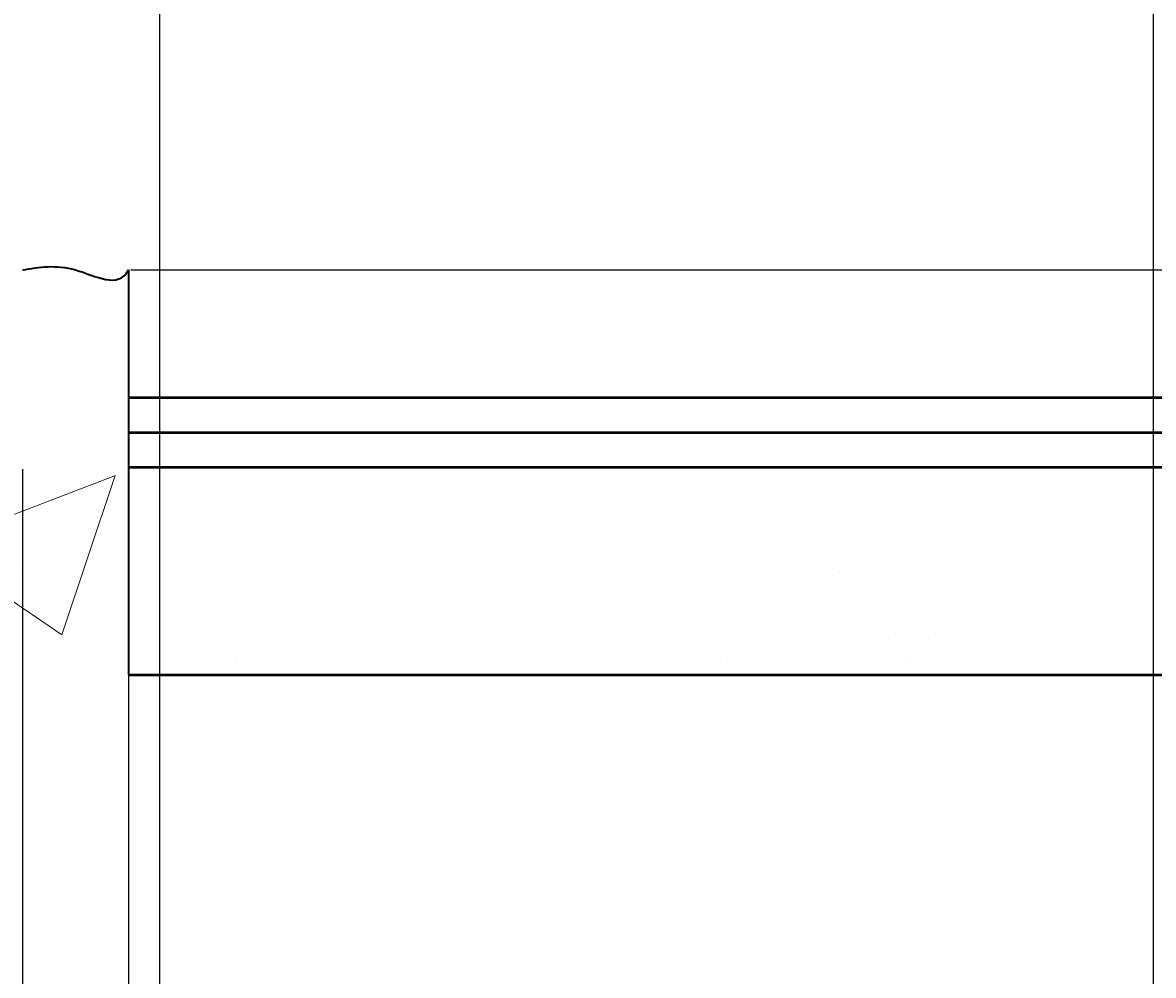
# Model space of a CAD drawing. Units: inches. Extents: x 2812 to 3051, y 1398 to 1659.
# Tile 10 of 65: x 2848 to 2880, y 1473 to 1501. Entities that reach past the tile are written whole.
import ezdxf

# ---------------------------------------------------------------- set-up
doc = ezdxf.new("R2010")
doc.units = ezdxf.units.IN
for name, color, linetype, lineweight in [('A-ANNO-DIMS', 2, 'Continuous', 18), ('P-SANR-PIPE', 4, 'Continuous', 35), ('S-CONC', 7, 'Continuous', 50), ('S-CONC-PATT', 8, 'Continuous', 18)]:
    doc.layers.add(name, color=color, linetype=linetype, lineweight=lineweight)
doc.styles.get("Standard").update_dxf_attribs({"font": 'arial.ttf'})
doc.dimstyles.get("Standard").update_dxf_attribs({"dimtxt": 0.18, "dimasz": 0.18, "dimexe": 0.18, "dimexo": 0.0625, "dimgap": 0.09, "dimtad": 0, "dimtih": 1, "dimtoh": 1, "dimdec": 4, "dimzin": 0, "dimdsep": 46, "dimtxsty": 'Standard', "dimcen": 0.09, "dimadec": 0, "dimazin": 0, "dimtfac": 1, "dimtdec": 4, "dimtofl": 0, "dimtmove": 0, "dimatfit": 3, "dimfxl": 1, "dimtolj": 1, "dimtzin": 0, "dimarcsym": 0})

# ---------------------------------------------------------------- blocks, each defined once
blk = doc.blocks.new('*D28')
at = {"layer": 'A-ANNO-DIMS', "color": 0, "lineweight": -2, "transparency": 16777216}
for p, q in [((2851.646, 1598.667), (2851.646, 1397.505)), ((2844.385, 1559.757), (2844.385, 1397.505)), ((2844.565, 1397.685), (2847.64, 1397.685)), ((2851.466, 1397.685), (2848.391, 1397.685))]:
    blk.add_line(p, q, dxfattribs=at)
at = {"layer": 'A-ANNO-DIMS', "color": 0, "transparency": 16777216}
for points in [[(2844.565, 1397.715), (2844.565, 1397.655), (2844.385, 1397.685)], [(2851.466, 1397.715), (2851.466, 1397.655), (2851.646, 1397.685)]]:
    blk.add_solid(points, dxfattribs=at)
at = {"layer": 'Defpoints', "color": 0, "transparency": 16777216}
for p in [(2851.646, 1598.73), (2844.385, 1559.82), (2851.646, 1397.685)]:
    blk.add_point(p, dxfattribs=at)
at = {"layer": 'A-ANNO-DIMS', "color": 0, "transparency": 16777216, "insert": (2848.016, 1397.685), "char_height": 0.18, "attachment_point": 5}
blk.add_mtext('\\A1;7.261', dxfattribs=at)
blk = doc.blocks.new('*D42')
at = {"layer": 'A-ANNO-DIMS', "color": 0, "lineweight": -2, "transparency": 16777216}
for p, q in [((2828.385, 1489.973), (2828.385, 1397.505)), ((2847.686, 1487.973), (2847.686, 1397.505)), ((2828.565, 1397.685), (2837.72, 1397.685)), ((2847.506, 1397.685), (2838.351, 1397.685))]:
    blk.add_line(p, q, dxfattribs=at)
at = {"layer": 'A-ANNO-DIMS', "color": 0, "transparency": 16777216}
for points in [[(2828.565, 1397.715), (2828.565, 1397.655), (2828.385, 1397.685)], [(2847.506, 1397.715), (2847.506, 1397.655), (2847.686, 1397.685)]]:
    blk.add_solid(points, dxfattribs=at)
at = {"layer": 'Defpoints', "color": 0, "transparency": 16777216}
for p in [(2828.385, 1490.035), (2847.686, 1488.035), (2847.686, 1397.685)]:
    blk.add_point(p, dxfattribs=at)
at = {"layer": 'A-ANNO-DIMS', "color": 0, "transparency": 16777216, "insert": (2838.036, 1397.685), "char_height": 0.18, "attachment_point": 5}
blk.add_mtext('\\A1;19.3', dxfattribs=at)
blk = doc.blocks.new('*D43')
at = {"layer": 'A-ANNO-DIMS', "color": 0, "lineweight": -2, "transparency": 16777216}
for p, q in [((2847.686, 1487.973), (2847.686, 1397.505)), ((2850.748, 1487.973), (2850.748, 1397.505)), ((2847.866, 1397.685), (2848.825, 1397.685)), ((2850.568, 1397.685), (2849.61, 1397.685))]:
    blk.add_line(p, q, dxfattribs=at)
at = {"layer": 'A-ANNO-DIMS', "color": 0, "transparency": 16777216}
for points in [[(2847.866, 1397.715), (2847.866, 1397.655), (2847.686, 1397.685)], [(2850.568, 1397.715), (2850.568, 1397.655), (2850.748, 1397.685)]]:
    blk.add_solid(points, dxfattribs=at)
at = {"layer": 'Defpoints', "color": 0, "transparency": 16777216}
for p in [(2847.686, 1488.035), (2850.748, 1488.035), (2850.748, 1397.685)]:
    blk.add_point(p, dxfattribs=at)
at = {"layer": 'A-ANNO-DIMS', "color": 0, "transparency": 16777216, "insert": (2849.217, 1397.685), "char_height": 0.18, "attachment_point": 5}
blk.add_mtext('\\A1;3.062', dxfattribs=at)
blk = doc.blocks.new('*D44')
at = {"layer": 'A-ANNO-DIMS', "color": 0, "lineweight": -2, "transparency": 16777216}
for p, q in [((2850.748, 1487.973), (2850.748, 1397.505)), ((2896.385, 1487.973), (2896.385, 1397.505)), ((2850.928, 1397.685), (2873.17, 1397.685)), ((2896.205, 1397.685), (2873.964, 1397.685))]:
    blk.add_line(p, q, dxfattribs=at)
at = {"layer": 'A-ANNO-DIMS', "color": 0, "transparency": 16777216}
for points in [[(2850.928, 1397.715), (2850.928, 1397.655), (2850.748, 1397.685)], [(2896.205, 1397.715), (2896.205, 1397.655), (2896.385, 1397.685)]]:
    blk.add_solid(points, dxfattribs=at)
at = {"layer": 'Defpoints', "color": 0, "transparency": 16777216}
for p in [(2850.748, 1488.035), (2896.385, 1488.035), (2896.385, 1397.685)]:
    blk.add_point(p, dxfattribs=at)
at = {"layer": 'A-ANNO-DIMS', "color": 0, "transparency": 16777216, "insert": (2873.567, 1397.685), "char_height": 0.18, "attachment_point": 5}
blk.add_mtext('\\A1;45.64', dxfattribs=at)
blk = doc.blocks.new('*D55')
at = {"layer": 'A-ANNO-DIMS', "color": 0, "lineweight": -2, "transparency": 16777216}
for p, q in [((2850.811, 1493.738), (3051.178, 1493.738)), ((3050.998, 1493.558), (3050.998, 1491.069)), ((3050.998, 1488.215), (3050.998, 1490.705)), ((2850.811, 1488.035), (3051.178, 1488.035))]:
    blk.add_line(p, q, dxfattribs=at)
at = {"layer": 'A-ANNO-DIMS', "color": 0, "transparency": 16777216}
for points in [[(3050.968, 1493.558), (3051.028, 1493.558), (3050.998, 1493.738)], [(3050.968, 1488.215), (3051.028, 1488.215), (3050.998, 1488.035)]]:
    blk.add_solid(points, dxfattribs=at)
at = {"layer": 'Defpoints', "color": 0, "transparency": 16777216}
for p in [(2850.748, 1493.738), (3050.998, 1493.738), (2850.748, 1488.035)]:
    blk.add_point(p, dxfattribs=at)
at = {"layer": 'A-ANNO-DIMS', "color": 0, "transparency": 16777216, "insert": (3050.998, 1490.887), "char_height": 0.18, "attachment_point": 5}
blk.add_mtext('\\A1;5.703', dxfattribs=at)
blk = doc.blocks.new('*D58')
at = {"layer": 'A-ANNO-DIMS', "color": 0, "lineweight": -2, "transparency": 16777216}
for p, q in [((2880.385, 1472.098), (2880.385, 1659.35)), ((2880.565, 1659.17), (2881.736, 1659.17)), ((2883.205, 1659.17), (2882.034, 1659.17)), ((2883.385, 1472.098), (2883.385, 1659.35))]:
    blk.add_line(p, q, dxfattribs=at)
at = {"layer": 'A-ANNO-DIMS', "color": 0, "transparency": 16777216}
for points in [[(2880.565, 1659.2), (2880.565, 1659.14), (2880.385, 1659.17)], [(2883.205, 1659.2), (2883.205, 1659.14), (2883.385, 1659.17)]]:
    blk.add_solid(points, dxfattribs=at)
at = {"layer": 'Defpoints', "color": 0, "transparency": 16777216}
for p in [(2883.385, 1659.17), (2880.385, 1472.035), (2883.385, 1472.035)]:
    blk.add_point(p, dxfattribs=at)
at = {"layer": 'A-ANNO-DIMS', "color": 0, "transparency": 16777216, "insert": (2881.885, 1659.17), "char_height": 0.18, "attachment_point": 5}
blk.add_mtext('\\A1;3', dxfattribs=at)

msp = doc.modelspace()

# ---------------------------------------------------------------- hatches: boundary and pattern name
at = {"layer": 'S-CONC-PATT'}
h = msp.add_hatch(dxfattribs=at)
h.set_pattern_fill('AR-SAND', color=256, scale=0.3)
h.paths.add_polyline_path([(3036.3849, 1416.0354), (3027.3849, 1416.0354), (2826.3849, 1416.0354), (2826.3849, 1410.0354), (2835.3849, 1410.0354), (3036.3849, 1410.0354)])
h.paths.add_polyline_path([(2970.3849, 1488.0354), (2969.3849, 1488.0354), (2941.3849, 1488.0354), (2941.3849, 1482.0354), (2970.3849, 1482.0354)])
h.paths.add_polyline_path([(3036.3849, 1488.0354), (3035.3849, 1488.0354), (3006.3849, 1488.0354), (3006.3849, 1482.0354), (3027.3849, 1482.0354), (3036.3849, 1482.0354)])
h.paths.add_polyline_path([(3034.3849, 1490.0354), (3008.3849, 1490.0354), (3008.3849, 1489.0354), (3034.3849, 1489.0354)])
h.paths.add_polyline_path([(3035.3849, 1489.0354), (3034.3849, 1489.0354), (3007.3849, 1489.0354), (3007.3849, 1488.0354), (3035.3849, 1488.0354)])
h.paths.add_polyline_path([(2968.3849, 1490.0354), (2943.3849, 1490.0354), (2943.3849, 1489.0354), (2968.3849, 1489.0354)])
h.paths.add_polyline_path([(2969.3849, 1489.0354), (2968.3849, 1489.0354), (2942.3849, 1489.0354), (2942.3849, 1488.0354), (2969.3849, 1488.0354)])
h.paths.add_polyline_path([(2896.3849, 1488.0354), (2826.3849, 1488.0354), (2826.3849, 1482.0354), (2896.3849, 1482.0354)])
h.paths.add_polyline_path([(2895.3849, 1489.0354), (2894.3849, 1489.0354), (2827.3849, 1489.0354), (2827.3849, 1488.0354), (2895.3849, 1488.0354)])
h.paths.add_polyline_path([(2894.3849, 1490.0354), (2828.3849, 1490.0354), (2828.3849, 1489.0354), (2894.3849, 1489.0354)])
h = msp.add_hatch(dxfattribs=at)
h.set_pattern_fill('AR-CONC', color=256, scale=0.3)
h.paths.add_polyline_path([(2896.3849, 1488.0354), (2826.3849, 1488.0354), (2826.3849, 1482.0354), (2896.3849, 1482.0354)])
h.paths.add_polyline_path([(2970.3849, 1488.0354), (2941.3849, 1488.0354), (2941.3849, 1482.0354), (2970.3849, 1482.0354)])
h.paths.add_polyline_path([(2968.3849, 1490.0354), (2943.3849, 1490.0354), (2943.3849, 1489.0354), (2968.3849, 1489.0354)])
h.paths.add_polyline_path([(2969.3849, 1489.0354), (2968.3849, 1489.0354), (2943.3849, 1489.0354), (2942.3849, 1489.0354), (2942.3849, 1488.0354), (2969.3849, 1488.0354)])
h.paths.add_polyline_path([(3036.3849, 1488.0354), (3035.3849, 1488.0354), (3006.3849, 1488.0354), (3006.3849, 1482.0354), (3027.3849, 1482.0354), (3036.3849, 1482.0354)])
h.paths.add_polyline_path([(3035.3849, 1489.0354), (3034.3849, 1489.0354), (3007.3849, 1489.0354), (3007.3849, 1488.0354), (3035.3849, 1488.0354)])
h.paths.add_polyline_path([(3034.3849, 1490.0354), (3008.3849, 1490.0354), (3008.3849, 1489.0354), (3034.3849, 1489.0354)])
h.paths.add_polyline_path([(2895.3849, 1489.0354), (2894.3849, 1489.0354), (2827.3849, 1489.0354), (2827.3849, 1488.0354), (2895.3849, 1488.0354)])
h.paths.add_polyline_path([(2894.3849, 1490.0354), (2828.3849, 1490.0354), (2828.3849, 1489.0354), (2894.3849, 1489.0354)])

# ---------------------------------------------------------------- linework, layer by layer
at = {"layer": 'P-SANR-PIPE'}
msp.add_line((2850.7485, 1493.7383), (2850.7485, 1482.0354), dxfattribs=at)
msp.add_open_spline([(2847.6863, 1493.7383), (2848.165, 1493.8196), (2849.1224, 1493.9821), (2850.4598, 1493.1692), (2850.7485, 1493.7383)], degree=3, dxfattribs=at)
at = {"layer": 'S-CONC'}
for p, q in [((3034.3849, 1490.0354), (2850.7485, 1490.0354)), ((2850.7485, 1489.0354), (3035.3849, 1489.0354)), ((2850.7485, 1488.0354), (3036.3849, 1488.0354)), ((2850.7485, 1482.0354), (3027.3849, 1482.0354))]:
    msp.add_line(p, q, dxfattribs=at)

# ---------------------------------------------------------------- dimensions: what is measured, and where the dimension line sits
at = {"layer": 'A-ANNO-DIMS'}
for base, p1, p2, override, picture, middle in [((2883.3849, 1659.17), (2880.3849, 1472.0354), (2883.3849, 1472.0354), {"dimdec": 0, "dimlfac": 1, "dimrnd": 0, "dimzin": 0, "dimdsep": 46, "dimlunit": 2}, '*D58', (2881.8849, 1659.17)), ((2851.6462, 1397.6854), (2844.3849, 1559.82), (2851.6462, 1598.7296), {"dimdec": 3, "dimlfac": 1, "dimrnd": 0, "dimzin": 0, "dimdsep": 46, "dimlunit": 2}, '*D28', (2848.0156, 1397.6854)), ((2847.6863, 1397.6854), (2828.3849, 1490.0354), (2847.6863, 1488.0354), {"dimdec": 1, "dimlfac": 1, "dimrnd": 0, "dimzin": 0, "dimdsep": 46, "dimlunit": 2}, '*D42', (2838.0356, 1397.6854)), ((2850.7485, 1397.6854), (2847.6863, 1488.0354), (2850.7485, 1488.0354), {"dimdec": 3, "dimlfac": 1, "dimrnd": 0, "dimzin": 0, "dimdsep": 46, "dimlunit": 2}, '*D43', (2849.2174, 1397.6854)), ((2896.3849, 1397.6854), (2850.7485, 1488.0354), (2896.3849, 1488.0354), {"dimdec": 2, "dimlfac": 1, "dimrnd": 0, "dimzin": 0, "dimdsep": 46, "dimlunit": 2}, '*D44', (2873.5667, 1397.6854))]:
    dim = msp.add_linear_dim(base=base, p1=p1, p2=p2, dimstyle='Standard', override=override, dxfattribs=at)
    dim.commit()
    dim.dimension.update_dxf_attribs({"geometry": picture, "text_midpoint": middle})
dim = msp.add_linear_dim(base=(3050.998, 1493.7383), p1=(2850.7485, 1488.0354), p2=(2850.7485, 1493.7383), angle=90, dimstyle='Standard', override={"dimdec": 3, "dimlfac": 1, "dimrnd": 0, "dimzin": 0, "dimdsep": 46, "dimlunit": 2}, dxfattribs=at)
dim.commit()
dim.dimension.update_dxf_attribs({"geometry": '*D55', "text_midpoint": (3050.998, 1490.8868)})

doc.saveas('drawing.dxf')
